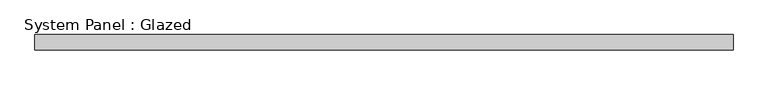
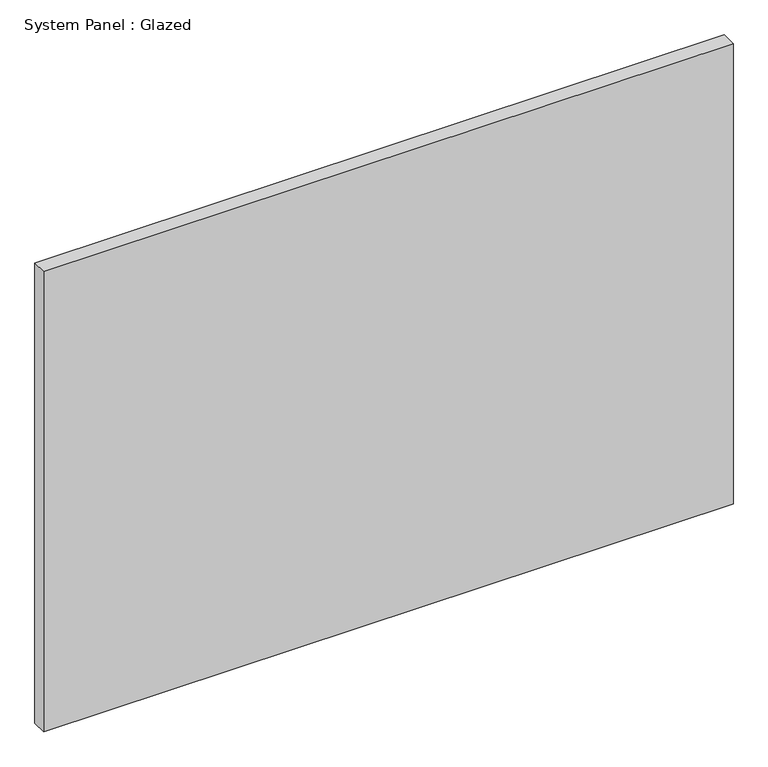
"""IFC4 building model written with IfcOpenShell, lengths in millimetres: plate geometry, System Panel : Glazed."""

from ifc_helpers import new_model, si_unit, origin, origin_with_axes, place, context, project, spatial, polyline, outline, extrude, source, transform, mapped, element, save


def system_panel_glazed_a4577834(model_context):
    return source(origin(), model_context, "Body", "SweptSolid", [
        extrude(outline(polyline([(581.0249999, 19.05), (-581.0249999, 19.05), (-581.0249999, 44.45), (581.0249999, 44.45), (581.0249999, 19.05)])), origin_with_axes(), (0.0, 0.0, 1.0), 820.4497825),
    ])


if __name__ == "__main__":
    model = new_model("IFC4")
    model_context = context("Model", 3, world=origin())
    ifc_project = project(units=[si_unit("LENGTHUNIT", "METRE", prefix="MILLI")], contexts=[model_context])
    site = spatial("IfcSite", under=ifc_project)
    building = spatial("IfcBuilding", under=site)
    placement = place(None, origin())
    system_panel_glazed_shape = system_panel_glazed_a4577834(model_context)
    element("IfcPlate", 1, ObjectType="System Panel : Glazed", at=placement, inside=building, context=model_context, shape_type="MappedRepresentation", body=[
        mapped(system_panel_glazed_shape, transform((0.0, 0.0, 0.0), x_axis=(1.0, 0.0, 0.0), y_axis=(0.0, 1.0, 0.0), z_axis=(0.0, 0.0, 1.0))),
    ])
    save(model, "model.ifc")

# Revit data of these elements
# Type "System Panel : Glazed"
#   Construction Type Id = "GSP4R"
#   Analytic Construction = "1/8 in Pilkington single glazing"
#   Visual Light Transmittance = 0.9
#   Solar Heat Gain Coefficient = 0.86
#   Heat Transfer Coefficient (U) = 1.18115 BTU/(h·ft²·°F)
#   Define Thermal Properties by = 1
# Element 1 (IfcPlate, "System Panel : Glazed")
#   Materials on its faces: "Glass"
# Materials
#   "Glass": class "Glass", colour RGB 0 128 192, transparency 0.75, Description = "Soda Lime Glass", Cost = 0
